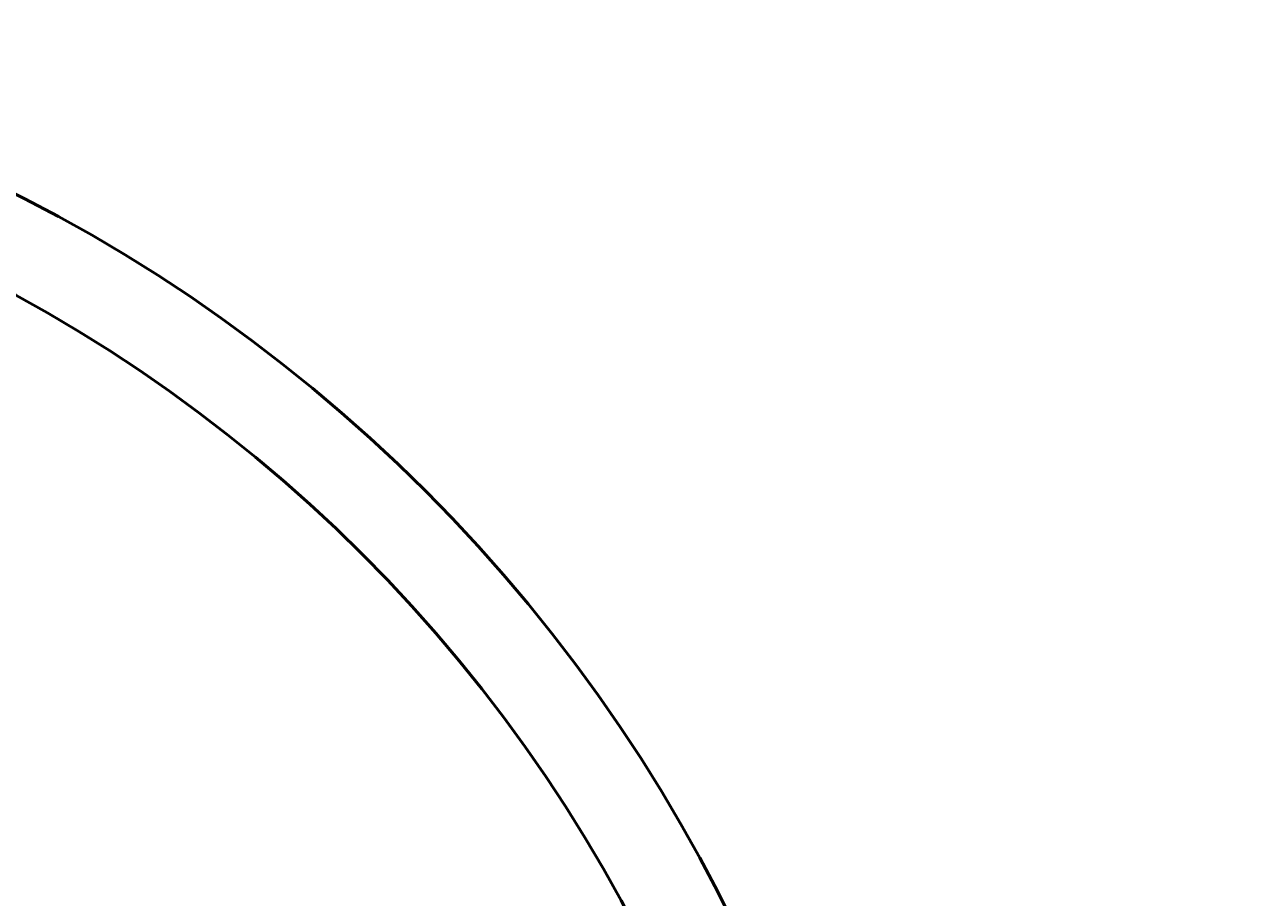
# Model space of a CAD drawing. Units: inches. Extents: x -99 to 284, y -92 to 134.
# Tile 12 of 16: x 72 to 140, y 55 to 104. Entities that reach past the tile are written whole.
import ezdxf

# ---------------------------------------------------------------- set-up
doc = ezdxf.new("R2010")
doc.units = ezdxf.units.IN
doc.header["$MEASUREMENT"] = 0
doc.layers.add('M-DIMS', color=2, linetype='Continuous', lineweight=18)
doc.layers.add('M-OUTL', color=7, linetype='Continuous', lineweight=50)
doc.styles.get("Standard").update_dxf_attribs({"font": 'arial.ttf'})
doc.dimstyles.get("Standard").update_dxf_attribs({"dimtxt": 0.18, "dimasz": 0.18, "dimexe": 0.18, "dimexo": 0.0625, "dimgap": 0.09, "dimtad": 0, "dimtih": 1, "dimtoh": 1, "dimdec": 4, "dimzin": 0, "dimdsep": 46, "dimtxsty": 'Standard', "dimcen": 0.09, "dimadec": 0, "dimazin": 0, "dimtfac": 1, "dimtdec": 4, "dimtofl": 0, "dimtmove": 0, "dimatfit": 3, "dimfxl": 1, "dimtolj": 1, "dimtzin": 0, "dimarcsym": 0})

# ---------------------------------------------------------------- blocks, each defined once
blk = doc.blocks.new('*D20')
at = {"layer": 'Defpoints', "color": 0, "transparency": 16777216}
for p in [(-35.23, 65.245), (99.183, -35.537)]:
    blk.add_point(p, dxfattribs=at)
at = {"layer": 'M-DIMS', "color": 0, "lineweight": -2, "transparency": 16777216}
for p, q in [((31.976, 14.764), (31.976, 14.944)), ((31.886, 14.854), (32.066, 14.854)), ((139.507, -65.772), (99.327, -35.645)), ((139.687, -65.772), (139.507, -65.772))]:
    blk.add_line(p, q, dxfattribs=at)
at = {"layer": 'M-DIMS', "color": 0, "transparency": 16777216}
blk.add_solid([(99.345, -35.621), (99.309, -35.669), (99.183, -35.537)], dxfattribs=at)
at = {"layer": 'M-DIMS', "color": 0, "transparency": 16777216, "insert": (140.074, -65.772), "char_height": 0.18, "attachment_point": 5}
blk.add_mtext('\\A1;∅168', dxfattribs=at)

msp = doc.modelspace()

# ---------------------------------------------------------------- linework, layer by layer
at = {"layer": 'M-OUTL'}
for radius in [89, 84]:
    msp.add_circle((31.9765, 14.8539), radius, dxfattribs=at)

# ---------------------------------------------------------------- dimensions: what is measured, and where the dimension line sits
at = {"layer": 'M-DIMS'}
dim = msp.add_diameter_dim_2p(p1=(-35.2301, 65.2451), p2=(99.1831, -35.5373), dimstyle='Standard', override={"dimdec": 0, "dimlfac": 1, "dimrnd": 0, "dimzin": 0, "dimdsep": 46, "dimlunit": 2}, dxfattribs=at)
dim.commit()
dim.dimension.update_dxf_attribs({"geometry": '*D20', "text_midpoint": (140.074, -65.772), "dimtype": 163})

doc.saveas('drawing.dxf')
